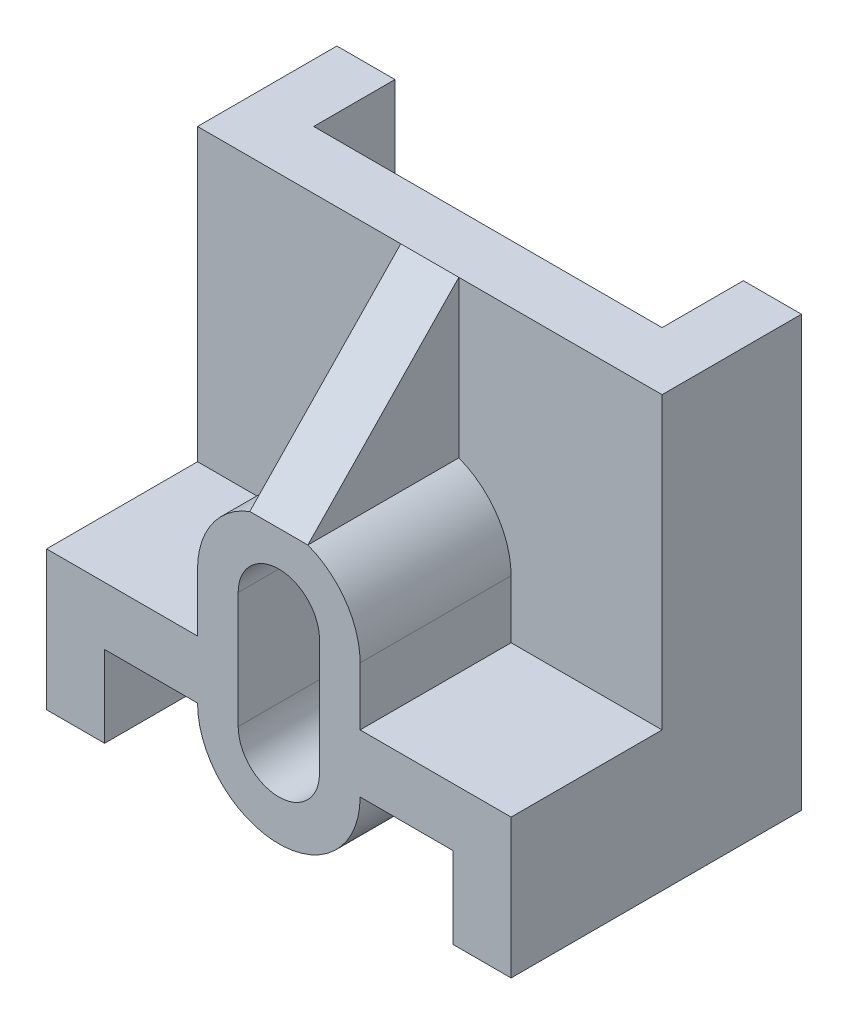
ISO-10303-21;
HEADER;
FILE_DESCRIPTION(('STEP AP214'),'2;1');
FILE_NAME('part.step','',(''),(''),'','','');
FILE_SCHEMA(('AUTOMOTIVE_DESIGN { 1 0 10303 214 1 1 1 1 }'));
ENDSEC;
DATA;
#1=APPLICATION_CONTEXT('core data for automotive mechanical design processes');
#2=APPLICATION_PROTOCOL_DEFINITION('international standard','automotive_design',2000,#1);
#3=PRODUCT_CONTEXT('',#1,'mechanical');
#4=PRODUCT('Part','Part','',(#3));
#5=PRODUCT_RELATED_PRODUCT_CATEGORY('part','',(#4));
#6=PRODUCT_DEFINITION_FORMATION('','',#4);
#7=PRODUCT_DEFINITION_CONTEXT('part definition',#1,'design');
#8=PRODUCT_DEFINITION('design','',#6,#7);
#9=PRODUCT_DEFINITION_SHAPE('','',#8);
#10=(LENGTH_UNIT() NAMED_UNIT(*) SI_UNIT(.MILLI.,.METRE.));
#11=(NAMED_UNIT(*) PLANE_ANGLE_UNIT() SI_UNIT($,.RADIAN.));
#12=(NAMED_UNIT(*) SI_UNIT($,.STERADIAN.) SOLID_ANGLE_UNIT());
#13=UNCERTAINTY_MEASURE_WITH_UNIT(LENGTH_MEASURE(1.E-05),#10,'distance_accuracy_value','');
#14=(GEOMETRIC_REPRESENTATION_CONTEXT(3) GLOBAL_UNCERTAINTY_ASSIGNED_CONTEXT((#13)) GLOBAL_UNIT_ASSIGNED_CONTEXT((#10,
#11,#12)) REPRESENTATION_CONTEXT('',''));
#15=CARTESIAN_POINT('',(0.,0.,0.));
#16=DIRECTION('',(0.,0.,1.));
#17=DIRECTION('',(1.,0.,0.));
#18=AXIS2_PLACEMENT_3D('',#15,#16,#17);
#19=CARTESIAN_POINT('',(0.,0.,0.));
#20=DIRECTION('',(0.,0.,-1.));
#21=DIRECTION('',(-1.,0.,0.));
#22=AXIS2_PLACEMENT_3D('',#19,#20,#21);
#23=PLANE('',#22);
#24=DIRECTION('',(0.,1.,0.));
#25=VECTOR('',#24,1.);
#26=CARTESIAN_POINT('',(47.,-10.,0.));
#27=LINE('',#26,#25);
#28=CARTESIAN_POINT('',(47.,-10.,0.));
#29=VERTEX_POINT('',#28);
#30=CARTESIAN_POINT('',(47.,10.,0.));
#31=VERTEX_POINT('',#30);
#32=EDGE_CURVE('E247',#29,#31,#27,.T.);
#33=ORIENTED_EDGE('',*,*,#32,.F.);
#34=CARTESIAN_POINT('',(40.,-10.,0.));
#35=DIRECTION('',(0.,0.,1.));
#36=DIRECTION('',(1.,0.,0.));
#37=AXIS2_PLACEMENT_3D('',#34,#35,#36);
#38=CIRCLE('',#37,7.);
#39=CARTESIAN_POINT('',(33.,-10.,0.));
#40=VERTEX_POINT('',#39);
#41=EDGE_CURVE('E64',#40,#29,#38,.T.);
#42=ORIENTED_EDGE('',*,*,#41,.F.);
#43=DIRECTION('',(0.,-1.,0.));
#44=VECTOR('',#43,1.);
#45=CARTESIAN_POINT('',(33.,-10.,0.));
#46=LINE('',#45,#44);
#47=CARTESIAN_POINT('',(33.,10.,0.));
#48=VERTEX_POINT('',#47);
#49=EDGE_CURVE('E258',#48,#40,#46,.T.);
#50=ORIENTED_EDGE('',*,*,#49,.F.);
#51=CARTESIAN_POINT('',(40.,10.,0.));
#52=DIRECTION('',(0.,0.,1.));
#53=DIRECTION('',(1.,0.,0.));
#54=AXIS2_PLACEMENT_3D('',#51,#52,#53);
#55=CIRCLE('',#54,7.);
#56=EDGE_CURVE('E251',#31,#48,#55,.T.);
#57=ORIENTED_EDGE('',*,*,#56,.F.);
#58=EDGE_LOOP('',(#33,#42,#50,#57));
#59=FACE_BOUND('',#58,.T.);
#60=DIRECTION('',(1.,0.,0.));
#61=VECTOR('',#60,1.);
#62=CARTESIAN_POINT('',(-114.874947873219,23.076696830622,0.));
#63=LINE('',#62,#61);
#64=CARTESIAN_POINT('',(35.,23.076696830622,0.));
#65=VERTEX_POINT('',#64);
#66=CARTESIAN_POINT('',(45.,23.076696830622,0.));
#67=VERTEX_POINT('',#66);
#68=EDGE_CURVE('E53',#65,#67,#63,.T.);
#69=ORIENTED_EDGE('',*,*,#68,.F.);
#70=CARTESIAN_POINT('',(40.,10.,0.));
#71=DIRECTION('',(0.,0.,1.));
#72=DIRECTION('',(1.,0.,0.));
#73=AXIS2_PLACEMENT_3D('',#70,#71,#72);
#74=CIRCLE('',#73,14.);
#75=CARTESIAN_POINT('',(26.,10.,0.));
#76=VERTEX_POINT('',#75);
#77=EDGE_CURVE('E282',#65,#76,#74,.T.);
#78=ORIENTED_EDGE('',*,*,#77,.T.);
#79=DIRECTION('',(0.,-1.,0.));
#80=VECTOR('',#79,1.);
#81=CARTESIAN_POINT('',(26.,10.,0.));
#82=LINE('',#81,#80);
#83=CARTESIAN_POINT('',(26.,0.,0.));
#84=VERTEX_POINT('',#83);
#85=EDGE_CURVE('E278',#76,#84,#82,.T.);
#86=ORIENTED_EDGE('',*,*,#85,.T.);
#87=DIRECTION('',(-1.,0.,0.));
#88=VECTOR('',#87,1.);
#89=CARTESIAN_POINT('',(0.,0.,0.));
#90=LINE('',#89,#88);
#91=CARTESIAN_POINT('',(0.,0.,0.));
#92=VERTEX_POINT('',#91);
#93=EDGE_CURVE('E374',#84,#92,#90,.T.);
#94=ORIENTED_EDGE('',*,*,#93,.T.);
#95=DIRECTION('',(0.,-1.,0.));
#96=VECTOR('',#95,1.);
#97=CARTESIAN_POINT('',(0.,-24.,0.));
#98=LINE('',#97,#96);
#99=CARTESIAN_POINT('',(0.,-24.,0.));
#100=VERTEX_POINT('',#99);
#101=EDGE_CURVE('E333',#92,#100,#98,.T.);
#102=ORIENTED_EDGE('',*,*,#101,.T.);
#103=DIRECTION('',(1.,0.,0.));
#104=VECTOR('',#103,1.);
#105=CARTESIAN_POINT('',(9.99999999999999,-24.,0.));
#106=LINE('',#105,#104);
#107=CARTESIAN_POINT('',(9.99999999999999,-24.,0.));
#108=VERTEX_POINT('',#107);
#109=EDGE_CURVE('E358',#100,#108,#106,.T.);
#110=ORIENTED_EDGE('',*,*,#109,.T.);
#111=DIRECTION('',(0.,1.,0.));
#112=VECTOR('',#111,1.);
#113=CARTESIAN_POINT('',(9.99999999999999,-10.,0.));
#114=LINE('',#113,#112);
#115=CARTESIAN_POINT('',(9.99999999999999,-10.,0.));
#116=VERTEX_POINT('',#115);
#117=EDGE_CURVE('E359',#108,#116,#114,.T.);
#118=ORIENTED_EDGE('',*,*,#117,.T.);
#119=DIRECTION('',(1.,0.,0.));
#120=VECTOR('',#119,1.);
#121=CARTESIAN_POINT('',(70.,-10.,0.));
#122=LINE('',#121,#120);
#123=CARTESIAN_POINT('',(26.,-10.,0.));
#124=VERTEX_POINT('',#123);
#125=EDGE_CURVE('E361',#116,#124,#122,.T.);
#126=ORIENTED_EDGE('',*,*,#125,.T.);
#127=CARTESIAN_POINT('',(40.,-10.,0.));
#128=DIRECTION('',(0.,0.,1.));
#129=DIRECTION('',(1.,0.,0.));
#130=AXIS2_PLACEMENT_3D('',#127,#128,#129);
#131=CIRCLE('',#130,14.);
#132=CARTESIAN_POINT('',(54.,-10.,0.));
#133=VERTEX_POINT('',#132);
#134=EDGE_CURVE('E281',#124,#133,#131,.T.);
#135=ORIENTED_EDGE('',*,*,#134,.T.);
#136=CARTESIAN_POINT('',(70.,-10.,0.));
#137=VERTEX_POINT('',#136);
#138=EDGE_CURVE('E362',#133,#137,#122,.T.);
#139=ORIENTED_EDGE('',*,*,#138,.T.);
#140=DIRECTION('',(0.,-1.,0.));
#141=VECTOR('',#140,1.);
#142=CARTESIAN_POINT('',(70.,-24.,0.));
#143=LINE('',#142,#141);
#144=CARTESIAN_POINT('',(70.,-24.,0.));
#145=VERTEX_POINT('',#144);
#146=EDGE_CURVE('E368',#137,#145,#143,.T.);
#147=ORIENTED_EDGE('',*,*,#146,.T.);
#148=DIRECTION('',(1.,0.,0.));
#149=VECTOR('',#148,1.);
#150=CARTESIAN_POINT('',(80.,-24.,0.));
#151=LINE('',#150,#149);
#152=CARTESIAN_POINT('',(80.,-24.,0.));
#153=VERTEX_POINT('',#152);
#154=EDGE_CURVE('E369',#145,#153,#151,.T.);
#155=ORIENTED_EDGE('',*,*,#154,.T.);
#156=DIRECTION('',(0.,1.,0.));
#157=VECTOR('',#156,1.);
#158=CARTESIAN_POINT('',(80.,0.,0.));
#159=LINE('',#158,#157);
#160=CARTESIAN_POINT('',(80.,0.,0.));
#161=VERTEX_POINT('',#160);
#162=EDGE_CURVE('E375',#153,#161,#159,.T.);
#163=ORIENTED_EDGE('',*,*,#162,.T.);
#164=CARTESIAN_POINT('',(54.,0.,0.));
#165=VERTEX_POINT('',#164);
#166=EDGE_CURVE('E338',#161,#165,#90,.T.);
#167=ORIENTED_EDGE('',*,*,#166,.T.);
#168=DIRECTION('',(0.,1.,0.));
#169=VECTOR('',#168,1.);
#170=CARTESIAN_POINT('',(54.,10.,0.));
#171=LINE('',#170,#169);
#172=CARTESIAN_POINT('',(54.,10.,0.));
#173=VERTEX_POINT('',#172);
#174=EDGE_CURVE('E288',#165,#173,#171,.T.);
#175=ORIENTED_EDGE('',*,*,#174,.T.);
#176=EDGE_CURVE('E279',#173,#67,#74,.T.);
#177=ORIENTED_EDGE('',*,*,#176,.T.);
#178=EDGE_LOOP('',(#69,#78,#86,#94,#102,#110,#118,#126,#135,#139,#147,#155,#163,#167,#175,#177));
#179=FACE_BOUND('',#178,.T.);
#180=ADVANCED_FACE('F39',(#59,#179),#23,.F.);
#181=CARTESIAN_POINT('',(0.,50.,0.));
#182=DIRECTION('',(0.,1.,0.));
#183=DIRECTION('',(0.,0.,1.));
#184=AXIS2_PLACEMENT_3D('',#181,#182,#183);
#185=PLANE('',#184);
#186=DIRECTION('',(1.,0.,0.));
#187=VECTOR('',#186,1.);
#188=CARTESIAN_POINT('',(0.,50.,-26.));
#189=LINE('',#188,#187);
#190=CARTESIAN_POINT('',(0.,50.,-26.));
#191=VERTEX_POINT('',#190);
#192=CARTESIAN_POINT('',(35.,50.,-26.));
#193=VERTEX_POINT('',#192);
#194=EDGE_CURVE('E227',#191,#193,#189,.T.);
#195=ORIENTED_EDGE('',*,*,#194,.T.);
#196=DIRECTION('',(1.,0.,0.));
#197=VECTOR('',#196,1.);
#198=CARTESIAN_POINT('',(-114.874947873219,50.,-26.));
#199=LINE('',#198,#197);
#200=CARTESIAN_POINT('',(45.,50.,-26.));
#201=VERTEX_POINT('',#200);
#202=EDGE_CURVE('E240',#193,#201,#199,.T.);
#203=ORIENTED_EDGE('',*,*,#202,.T.);
#204=CARTESIAN_POINT('',(80.,50.,-26.));
#205=VERTEX_POINT('',#204);
#206=EDGE_CURVE('E212',#201,#205,#189,.T.);
#207=ORIENTED_EDGE('',*,*,#206,.T.);
#208=DIRECTION('',(0.,0.,-1.));
#209=VECTOR('',#208,1.);
#210=CARTESIAN_POINT('',(80.,50.,-50.));
#211=LINE('',#210,#209);
#212=CARTESIAN_POINT('',(80.,50.,-50.));
#213=VERTEX_POINT('',#212);
#214=EDGE_CURVE('E323',#205,#213,#211,.T.);
#215=ORIENTED_EDGE('',*,*,#214,.T.);
#216=DIRECTION('',(-1.,0.,0.));
#217=VECTOR('',#216,1.);
#218=CARTESIAN_POINT('',(0.,50.,-50.));
#219=LINE('',#218,#217);
#220=CARTESIAN_POINT('',(70.,50.,-50.));
#221=VERTEX_POINT('',#220);
#222=EDGE_CURVE('E326',#213,#221,#219,.T.);
#223=ORIENTED_EDGE('',*,*,#222,.T.);
#224=DIRECTION('',(0.,0.,-1.));
#225=VECTOR('',#224,1.);
#226=CARTESIAN_POINT('',(70.,50.,-50.));
#227=LINE('',#226,#225);
#228=CARTESIAN_POINT('',(70.,50.,-36.));
#229=VERTEX_POINT('',#228);
#230=EDGE_CURVE('E306',#229,#221,#227,.T.);
#231=ORIENTED_EDGE('',*,*,#230,.F.);
#232=DIRECTION('',(1.,0.,0.));
#233=VECTOR('',#232,1.);
#234=CARTESIAN_POINT('',(10.,50.,-36.));
#235=LINE('',#234,#233);
#236=CARTESIAN_POINT('',(10.,50.,-36.));
#237=VERTEX_POINT('',#236);
#238=EDGE_CURVE('E302',#237,#229,#235,.T.);
#239=ORIENTED_EDGE('',*,*,#238,.F.);
#240=DIRECTION('',(0.,0.,1.));
#241=VECTOR('',#240,1.);
#242=CARTESIAN_POINT('',(9.99999999999999,50.,-50.));
#243=LINE('',#242,#241);
#244=CARTESIAN_POINT('',(9.99999999999999,50.,-50.));
#245=VERTEX_POINT('',#244);
#246=EDGE_CURVE('E301',#245,#237,#243,.T.);
#247=ORIENTED_EDGE('',*,*,#246,.F.);
#248=CARTESIAN_POINT('',(0.,50.,-50.));
#249=VERTEX_POINT('',#248);
#250=EDGE_CURVE('E324',#245,#249,#219,.T.);
#251=ORIENTED_EDGE('',*,*,#250,.T.);
#252=DIRECTION('',(0.,0.,1.));
#253=VECTOR('',#252,1.);
#254=CARTESIAN_POINT('',(0.,50.,-50.));
#255=LINE('',#254,#253);
#256=EDGE_CURVE('E229',#249,#191,#255,.T.);
#257=ORIENTED_EDGE('',*,*,#256,.T.);
#258=EDGE_LOOP('',(#195,#203,#207,#215,#223,#231,#239,#247,#251,#257));
#259=FACE_BOUND('',#258,.T.);
#260=ADVANCED_FACE('F236',(#259),#185,.T.);
#261=CARTESIAN_POINT('',(35.,50.,0.));
#262=DIRECTION('',(1.,0.,0.));
#263=DIRECTION('',(0.,1.,0.));
#264=AXIS2_PLACEMENT_3D('',#261,#262,#263);
#265=PLANE('',#264);
#266=DIRECTION('',(0.,0.719333547480298,-0.694664845425051));
#267=VECTOR('',#266,1.);
#268=CARTESIAN_POINT('',(35.,50.,-26.));
#269=LINE('',#268,#267);
#270=EDGE_CURVE('E241',#65,#193,#269,.T.);
#271=ORIENTED_EDGE('',*,*,#270,.T.);
#272=DIRECTION('',(0.,-1.,0.));
#273=VECTOR('',#272,1.);
#274=CARTESIAN_POINT('',(35.,50.,-26.));
#275=LINE('',#274,#273);
#276=CARTESIAN_POINT('',(35.,23.076696830622,-26.));
#277=VERTEX_POINT('',#276);
#278=EDGE_CURVE('E231',#193,#277,#275,.T.);
#279=ORIENTED_EDGE('',*,*,#278,.T.);
#280=DIRECTION('',(0.,0.,1.));
#281=VECTOR('',#280,1.);
#282=CARTESIAN_POINT('',(35.,23.076696830622,-26.));
#283=LINE('',#282,#281);
#284=EDGE_CURVE('E50',#65,#277,#283,.F.);
#285=ORIENTED_EDGE('',*,*,#284,.F.);
#286=EDGE_LOOP('',(#271,#279,#285));
#287=FACE_BOUND('',#286,.T.);
#288=ADVANCED_FACE('F499',(#287),#265,.F.);
#289=CARTESIAN_POINT('',(45.,50.,0.));
#290=DIRECTION('',(-1.,0.,0.));
#291=DIRECTION('',(0.,0.,1.));
#292=AXIS2_PLACEMENT_3D('',#289,#290,#291);
#293=PLANE('',#292);
#294=DIRECTION('',(0.,0.719333547480298,-0.694664845425051));
#295=VECTOR('',#294,1.);
#296=CARTESIAN_POINT('',(45.,37.0079110831942,-13.4534595657953));
#297=LINE('',#296,#295);
#298=EDGE_CURVE('E11',#67,#201,#297,.T.);
#299=ORIENTED_EDGE('',*,*,#298,.F.);
#300=DIRECTION('',(0.,0.,1.));
#301=VECTOR('',#300,1.);
#302=CARTESIAN_POINT('',(45.,23.076696830622,-26.));
#303=LINE('',#302,#301);
#304=CARTESIAN_POINT('',(45.,23.076696830622,-26.));
#305=VERTEX_POINT('',#304);
#306=EDGE_CURVE('E235',#305,#67,#303,.T.);
#307=ORIENTED_EDGE('',*,*,#306,.F.);
#308=DIRECTION('',(0.,1.,0.));
#309=VECTOR('',#308,1.);
#310=CARTESIAN_POINT('',(45.,50.,-26.));
#311=LINE('',#310,#309);
#312=EDGE_CURVE('E217',#305,#201,#311,.T.);
#313=ORIENTED_EDGE('',*,*,#312,.T.);
#314=EDGE_LOOP('',(#299,#307,#313));
#315=FACE_BOUND('',#314,.T.);
#316=ADVANCED_FACE('F228',(#315),#293,.F.);
#317=CARTESIAN_POINT('',(0.,50.,-26.));
#318=DIRECTION('',(0.,0.,-1.));
#319=DIRECTION('',(-1.,0.,0.));
#320=AXIS2_PLACEMENT_3D('',#317,#318,#319);
#321=PLANE('',#320);
#322=ORIENTED_EDGE('',*,*,#278,.F.);
#323=ORIENTED_EDGE('',*,*,#194,.F.);
#324=DIRECTION('',(0.,-1.,0.));
#325=VECTOR('',#324,1.);
#326=CARTESIAN_POINT('',(0.,50.,-26.));
#327=LINE('',#326,#325);
#328=CARTESIAN_POINT('',(0.,0.,-26.));
#329=VERTEX_POINT('',#328);
#330=EDGE_CURVE('E335',#191,#329,#327,.T.);
#331=ORIENTED_EDGE('',*,*,#330,.T.);
#332=DIRECTION('',(1.,0.,0.));
#333=VECTOR('',#332,1.);
#334=CARTESIAN_POINT('',(0.,0.,-26.));
#335=LINE('',#334,#333);
#336=CARTESIAN_POINT('',(26.,0.,-26.));
#337=VERTEX_POINT('',#336);
#338=EDGE_CURVE('E321',#329,#337,#335,.T.);
#339=ORIENTED_EDGE('',*,*,#338,.T.);
#340=DIRECTION('',(0.,-1.,0.));
#341=VECTOR('',#340,1.);
#342=CARTESIAN_POINT('',(26.,10.,-26.));
#343=LINE('',#342,#341);
#344=CARTESIAN_POINT('',(26.,10.,-26.));
#345=VERTEX_POINT('',#344);
#346=EDGE_CURVE('E271',#345,#337,#343,.T.);
#347=ORIENTED_EDGE('',*,*,#346,.F.);
#348=CARTESIAN_POINT('',(40.,10.,-26.));
#349=DIRECTION('',(0.,0.,1.));
#350=DIRECTION('',(1.,0.,0.));
#351=AXIS2_PLACEMENT_3D('',#348,#349,#350);
#352=CIRCLE('',#351,14.);
#353=EDGE_CURVE('E275',#277,#345,#352,.T.);
#354=ORIENTED_EDGE('',*,*,#353,.F.);
#355=EDGE_LOOP('',(#322,#323,#331,#339,#347,#354));
#356=FACE_BOUND('',#355,.T.);
#357=ADVANCED_FACE('F424',(#356),#321,.F.);
#358=ORIENTED_EDGE('',*,*,#312,.F.);
#359=CARTESIAN_POINT('',(54.,10.,-26.));
#360=VERTEX_POINT('',#359);
#361=EDGE_CURVE('E267',#360,#305,#352,.T.);
#362=ORIENTED_EDGE('',*,*,#361,.F.);
#363=DIRECTION('',(0.,-1.,0.));
#364=VECTOR('',#363,1.);
#365=CARTESIAN_POINT('',(54.,50.,-26.));
#366=LINE('',#365,#364);
#367=CARTESIAN_POINT('',(54.,0.,-26.));
#368=VERTEX_POINT('',#367);
#369=EDGE_CURVE('E381',#360,#368,#366,.T.);
#370=ORIENTED_EDGE('',*,*,#369,.T.);
#371=CARTESIAN_POINT('',(80.,0.,-26.));
#372=VERTEX_POINT('',#371);
#373=EDGE_CURVE('E319',#368,#372,#335,.T.);
#374=ORIENTED_EDGE('',*,*,#373,.T.);
#375=DIRECTION('',(0.,-1.,0.));
#376=VECTOR('',#375,1.);
#377=CARTESIAN_POINT('',(80.,50.,-26.));
#378=LINE('',#377,#376);
#379=EDGE_CURVE('E222',#205,#372,#378,.T.);
#380=ORIENTED_EDGE('',*,*,#379,.F.);
#381=ORIENTED_EDGE('',*,*,#206,.F.);
#382=EDGE_LOOP('',(#358,#362,#370,#374,#380,#381));
#383=FACE_BOUND('',#382,.T.);
#384=ADVANCED_FACE('F216',(#383),#321,.F.);
#385=CARTESIAN_POINT('',(40.,10.,-26.));
#386=DIRECTION('',(0.,0.,1.));
#387=DIRECTION('',(1.,0.,0.));
#388=AXIS2_PLACEMENT_3D('',#385,#386,#387);
#389=CYLINDRICAL_SURFACE('',#388,14.);
#390=ORIENTED_EDGE('',*,*,#77,.F.);
#391=ORIENTED_EDGE('',*,*,#284,.T.);
#392=ORIENTED_EDGE('',*,*,#353,.T.);
#393=DIRECTION('',(0.,0.,1.));
#394=VECTOR('',#393,1.);
#395=CARTESIAN_POINT('',(26.,10.,-26.));
#396=LINE('',#395,#394);
#397=EDGE_CURVE('E280',#345,#76,#396,.T.);
#398=ORIENTED_EDGE('',*,*,#397,.T.);
#399=EDGE_LOOP('',(#390,#391,#392,#398));
#400=FACE_BOUND('',#399,.T.);
#401=ADVANCED_FACE('F416',(#400),#389,.T.);
#402=ORIENTED_EDGE('',*,*,#361,.T.);
#403=ORIENTED_EDGE('',*,*,#306,.T.);
#404=ORIENTED_EDGE('',*,*,#176,.F.);
#405=DIRECTION('',(0.,0.,1.));
#406=VECTOR('',#405,1.);
#407=CARTESIAN_POINT('',(54.,10.,-26.));
#408=LINE('',#407,#406);
#409=EDGE_CURVE('E286',#360,#173,#408,.T.);
#410=ORIENTED_EDGE('',*,*,#409,.F.);
#411=EDGE_LOOP('',(#402,#403,#404,#410));
#412=FACE_BOUND('',#411,.T.);
#413=ADVANCED_FACE('F544',(#412),#389,.T.);
#414=CARTESIAN_POINT('',(70.,-10.,-50.));
#415=DIRECTION('',(0.,-1.,0.));
#416=DIRECTION('',(0.,0.,-1.));
#417=AXIS2_PLACEMENT_3D('',#414,#415,#416);
#418=PLANE('',#417);
#419=DIRECTION('',(0.,0.,1.));
#420=VECTOR('',#419,1.);
#421=CARTESIAN_POINT('',(33.,-10.,-50.));
#422=LINE('',#421,#420);
#423=CARTESIAN_POINT('',(33.,-10.,-36.));
#424=VERTEX_POINT('',#423);
#425=CARTESIAN_POINT('',(33.,-10.,-26.));
#426=VERTEX_POINT('',#425);
#427=EDGE_CURVE('E265',#424,#426,#422,.T.);
#428=ORIENTED_EDGE('',*,*,#427,.T.);
#429=DIRECTION('',(-1.,0.,0.));
#430=VECTOR('',#429,1.);
#431=CARTESIAN_POINT('',(70.,-10.,-26.));
#432=LINE('',#431,#430);
#433=CARTESIAN_POINT('',(26.,-10.,-26.));
#434=VERTEX_POINT('',#433);
#435=EDGE_CURVE('E396',#426,#434,#432,.T.);
#436=ORIENTED_EDGE('',*,*,#435,.T.);
#437=DIRECTION('',(0.,0.,1.));
#438=VECTOR('',#437,1.);
#439=CARTESIAN_POINT('',(26.,-10.,-26.));
#440=LINE('',#439,#438);
#441=EDGE_CURVE('E293',#434,#124,#440,.T.);
#442=ORIENTED_EDGE('',*,*,#441,.T.);
#443=ORIENTED_EDGE('',*,*,#125,.F.);
#444=DIRECTION('',(0.,0.,1.));
#445=VECTOR('',#444,1.);
#446=CARTESIAN_POINT('',(9.99999999999999,-10.,-50.));
#447=LINE('',#446,#445);
#448=CARTESIAN_POINT('',(10.,-10.,-36.));
#449=VERTEX_POINT('',#448);
#450=EDGE_CURVE('E392',#449,#116,#447,.T.);
#451=ORIENTED_EDGE('',*,*,#450,.F.);
#452=DIRECTION('',(-1.,0.,0.));
#453=VECTOR('',#452,1.);
#454=CARTESIAN_POINT('',(70.,-10.,-36.));
#455=LINE('',#454,#453);
#456=EDGE_CURVE('E314',#424,#449,#455,.T.);
#457=ORIENTED_EDGE('',*,*,#456,.F.);
#458=EDGE_LOOP('',(#428,#436,#442,#443,#451,#457));
#459=FACE_BOUND('',#458,.T.);
#460=ADVANCED_FACE('F437',(#459),#418,.T.);
#461=CARTESIAN_POINT('',(0.,0.,-50.));
#462=DIRECTION('',(0.,1.,0.));
#463=DIRECTION('',(0.,0.,1.));
#464=AXIS2_PLACEMENT_3D('',#461,#462,#463);
#465=PLANE('',#464);
#466=DIRECTION('',(0.,0.,-1.));
#467=VECTOR('',#466,1.);
#468=CARTESIAN_POINT('',(54.,0.,-50.));
#469=LINE('',#468,#467);
#470=EDGE_CURVE('E303',#165,#368,#469,.T.);
#471=ORIENTED_EDGE('',*,*,#470,.F.);
#472=ORIENTED_EDGE('',*,*,#166,.F.);
#473=DIRECTION('',(0.,0.,1.));
#474=VECTOR('',#473,1.);
#475=CARTESIAN_POINT('',(80.,0.,-50.));
#476=LINE('',#475,#474);
#477=EDGE_CURVE('E385',#372,#161,#476,.T.);
#478=ORIENTED_EDGE('',*,*,#477,.F.);
#479=ORIENTED_EDGE('',*,*,#373,.F.);
#480=EDGE_LOOP('',(#471,#472,#478,#479));
#481=FACE_BOUND('',#480,.T.);
#482=ADVANCED_FACE('F510',(#481),#465,.T.);
#483=CARTESIAN_POINT('',(0.,0.,-50.));
#484=DIRECTION('',(0.,0.,-1.));
#485=DIRECTION('',(-1.,0.,0.));
#486=AXIS2_PLACEMENT_3D('',#483,#484,#485);
#487=PLANE('',#486);
#488=ORIENTED_EDGE('',*,*,#250,.F.);
#489=DIRECTION('',(0.,1.,0.));
#490=VECTOR('',#489,1.);
#491=CARTESIAN_POINT('',(9.99999999999999,-10.,-50.));
#492=LINE('',#491,#490);
#493=CARTESIAN_POINT('',(9.99999999999999,-24.,-50.));
#494=VERTEX_POINT('',#493);
#495=EDGE_CURVE('E341',#494,#245,#492,.T.);
#496=ORIENTED_EDGE('',*,*,#495,.F.);
#497=DIRECTION('',(1.,0.,0.));
#498=VECTOR('',#497,1.);
#499=CARTESIAN_POINT('',(9.99999999999999,-24.,-50.));
#500=LINE('',#499,#498);
#501=CARTESIAN_POINT('',(0.,-24.,-50.));
#502=VERTEX_POINT('',#501);
#503=EDGE_CURVE('E336',#502,#494,#500,.T.);
#504=ORIENTED_EDGE('',*,*,#503,.F.);
#505=DIRECTION('',(0.,-1.,0.));
#506=VECTOR('',#505,1.);
#507=CARTESIAN_POINT('',(0.,-24.,-50.));
#508=LINE('',#507,#506);
#509=EDGE_CURVE('E337',#249,#502,#508,.T.);
#510=ORIENTED_EDGE('',*,*,#509,.F.);
#511=EDGE_LOOP('',(#488,#496,#504,#510));
#512=FACE_BOUND('',#511,.T.);
#513=ADVANCED_FACE('F527',(#512),#487,.T.);
#514=CARTESIAN_POINT('',(0.,-24.,-50.));
#515=DIRECTION('',(-1.,0.,0.));
#516=DIRECTION('',(0.,0.,1.));
#517=AXIS2_PLACEMENT_3D('',#514,#515,#516);
#518=PLANE('',#517);
#519=ORIENTED_EDGE('',*,*,#101,.F.);
#520=DIRECTION('',(0.,0.,1.));
#521=VECTOR('',#520,1.);
#522=CARTESIAN_POINT('',(0.,0.,-50.));
#523=LINE('',#522,#521);
#524=EDGE_CURVE('E378',#329,#92,#523,.T.);
#525=ORIENTED_EDGE('',*,*,#524,.F.);
#526=ORIENTED_EDGE('',*,*,#330,.F.);
#527=ORIENTED_EDGE('',*,*,#256,.F.);
#528=ORIENTED_EDGE('',*,*,#509,.T.);
#529=DIRECTION('',(0.,0.,1.));
#530=VECTOR('',#529,1.);
#531=CARTESIAN_POINT('',(0.,-24.,-50.));
#532=LINE('',#531,#530);
#533=EDGE_CURVE('E355',#502,#100,#532,.T.);
#534=ORIENTED_EDGE('',*,*,#533,.T.);
#535=EDGE_LOOP('',(#519,#525,#526,#527,#528,#534));
#536=FACE_BOUND('',#535,.T.);
#537=ADVANCED_FACE('F41',(#536),#518,.T.);
#538=DIRECTION('',(0.,0.,1.));
#539=VECTOR('',#538,1.);
#540=CARTESIAN_POINT('',(26.,0.,-50.));
#541=LINE('',#540,#539);
#542=EDGE_CURVE('E292',#337,#84,#541,.T.);
#543=ORIENTED_EDGE('',*,*,#542,.F.);
#544=ORIENTED_EDGE('',*,*,#338,.F.);
#545=ORIENTED_EDGE('',*,*,#524,.T.);
#546=ORIENTED_EDGE('',*,*,#93,.F.);
#547=EDGE_LOOP('',(#543,#544,#545,#546));
#548=FACE_BOUND('',#547,.T.);
#549=ADVANCED_FACE('F431',(#548),#465,.T.);
#550=CARTESIAN_POINT('',(80.,0.,-50.));
#551=DIRECTION('',(1.,0.,0.));
#552=DIRECTION('',(0.,0.,-1.));
#553=AXIS2_PLACEMENT_3D('',#550,#551,#552);
#554=PLANE('',#553);
#555=ORIENTED_EDGE('',*,*,#162,.F.);
#556=DIRECTION('',(0.,0.,1.));
#557=VECTOR('',#556,1.);
#558=CARTESIAN_POINT('',(80.,-24.,-50.));
#559=LINE('',#558,#557);
#560=CARTESIAN_POINT('',(80.,-24.,-50.));
#561=VERTEX_POINT('',#560);
#562=EDGE_CURVE('E383',#561,#153,#559,.T.);
#563=ORIENTED_EDGE('',*,*,#562,.F.);
#564=DIRECTION('',(0.,1.,0.));
#565=VECTOR('',#564,1.);
#566=CARTESIAN_POINT('',(80.,0.,-50.));
#567=LINE('',#566,#565);
#568=EDGE_CURVE('E352',#561,#213,#567,.T.);
#569=ORIENTED_EDGE('',*,*,#568,.T.);
#570=ORIENTED_EDGE('',*,*,#214,.F.);
#571=ORIENTED_EDGE('',*,*,#379,.T.);
#572=ORIENTED_EDGE('',*,*,#477,.T.);
#573=EDGE_LOOP('',(#555,#563,#569,#570,#571,#572));
#574=FACE_BOUND('',#573,.T.);
#575=ADVANCED_FACE('F508',(#574),#554,.T.);
#576=CARTESIAN_POINT('',(80.,-24.,-50.));
#577=DIRECTION('',(0.,-1.,0.));
#578=DIRECTION('',(0.,0.,-1.));
#579=AXIS2_PLACEMENT_3D('',#576,#577,#578);
#580=PLANE('',#579);
#581=ORIENTED_EDGE('',*,*,#154,.F.);
#582=DIRECTION('',(0.,0.,1.));
#583=VECTOR('',#582,1.);
#584=CARTESIAN_POINT('',(70.,-24.,-50.));
#585=LINE('',#584,#583);
#586=CARTESIAN_POINT('',(70.,-24.,-50.));
#587=VERTEX_POINT('',#586);
#588=EDGE_CURVE('E387',#587,#145,#585,.T.);
#589=ORIENTED_EDGE('',*,*,#588,.F.);
#590=DIRECTION('',(1.,0.,0.));
#591=VECTOR('',#590,1.);
#592=CARTESIAN_POINT('',(80.,-24.,-50.));
#593=LINE('',#592,#591);
#594=EDGE_CURVE('E346',#587,#561,#593,.T.);
#595=ORIENTED_EDGE('',*,*,#594,.T.);
#596=ORIENTED_EDGE('',*,*,#562,.T.);
#597=EDGE_LOOP('',(#581,#589,#595,#596));
#598=FACE_BOUND('',#597,.T.);
#599=ADVANCED_FACE('F507',(#598),#580,.T.);
#600=CARTESIAN_POINT('',(70.,-24.,-50.));
#601=DIRECTION('',(-1.,0.,0.));
#602=DIRECTION('',(0.,0.,1.));
#603=AXIS2_PLACEMENT_3D('',#600,#601,#602);
#604=PLANE('',#603);
#605=DIRECTION('',(0.,0.,1.));
#606=VECTOR('',#605,1.);
#607=CARTESIAN_POINT('',(70.,-10.,-50.));
#608=LINE('',#607,#606);
#609=CARTESIAN_POINT('',(70.,-10.,-36.));
#610=VERTEX_POINT('',#609);
#611=EDGE_CURVE('E389',#610,#137,#608,.T.);
#612=ORIENTED_EDGE('',*,*,#611,.F.);
#613=DIRECTION('',(0.,1.,0.));
#614=VECTOR('',#613,1.);
#615=CARTESIAN_POINT('',(70.,-24.,-36.));
#616=LINE('',#615,#614);
#617=EDGE_CURVE('E315',#610,#229,#616,.T.);
#618=ORIENTED_EDGE('',*,*,#617,.T.);
#619=ORIENTED_EDGE('',*,*,#230,.T.);
#620=DIRECTION('',(0.,-1.,0.));
#621=VECTOR('',#620,1.);
#622=CARTESIAN_POINT('',(70.,-24.,-50.));
#623=LINE('',#622,#621);
#624=EDGE_CURVE('E342',#221,#587,#623,.T.);
#625=ORIENTED_EDGE('',*,*,#624,.T.);
#626=ORIENTED_EDGE('',*,*,#588,.T.);
#627=ORIENTED_EDGE('',*,*,#146,.F.);
#628=EDGE_LOOP('',(#612,#618,#619,#625,#626,#627));
#629=FACE_BOUND('',#628,.T.);
#630=ADVANCED_FACE('F473',(#629),#604,.T.);
#631=DIRECTION('',(0.,0.,1.));
#632=VECTOR('',#631,1.);
#633=CARTESIAN_POINT('',(47.,-10.,-50.));
#634=LINE('',#633,#632);
#635=CARTESIAN_POINT('',(47.,-10.,-36.));
#636=VERTEX_POINT('',#635);
#637=CARTESIAN_POINT('',(47.,-10.,-26.));
#638=VERTEX_POINT('',#637);
#639=EDGE_CURVE('E270',#636,#638,#634,.T.);
#640=ORIENTED_EDGE('',*,*,#639,.F.);
#641=EDGE_CURVE('E320',#610,#636,#455,.T.);
#642=ORIENTED_EDGE('',*,*,#641,.F.);
#643=ORIENTED_EDGE('',*,*,#611,.T.);
#644=ORIENTED_EDGE('',*,*,#138,.F.);
#645=DIRECTION('',(0.,0.,1.));
#646=VECTOR('',#645,1.);
#647=CARTESIAN_POINT('',(54.,-10.,-26.));
#648=LINE('',#647,#646);
#649=CARTESIAN_POINT('',(54.,-10.,-26.));
#650=VERTEX_POINT('',#649);
#651=EDGE_CURVE('E295',#650,#133,#648,.T.);
#652=ORIENTED_EDGE('',*,*,#651,.F.);
#653=EDGE_CURVE('E399',#650,#638,#432,.T.);
#654=ORIENTED_EDGE('',*,*,#653,.T.);
#655=EDGE_LOOP('',(#640,#642,#643,#644,#652,#654));
#656=FACE_BOUND('',#655,.T.);
#657=ADVANCED_FACE('F455',(#656),#418,.T.);
#658=CARTESIAN_POINT('',(9.99999999999999,-10.,-50.));
#659=DIRECTION('',(1.,0.,0.));
#660=DIRECTION('',(0.,0.,-1.));
#661=AXIS2_PLACEMENT_3D('',#658,#659,#660);
#662=PLANE('',#661);
#663=ORIENTED_EDGE('',*,*,#117,.F.);
#664=DIRECTION('',(0.,0.,1.));
#665=VECTOR('',#664,1.);
#666=CARTESIAN_POINT('',(9.99999999999999,-24.,-50.));
#667=LINE('',#666,#665);
#668=EDGE_CURVE('E395',#494,#108,#667,.T.);
#669=ORIENTED_EDGE('',*,*,#668,.F.);
#670=ORIENTED_EDGE('',*,*,#495,.T.);
#671=ORIENTED_EDGE('',*,*,#246,.T.);
#672=DIRECTION('',(0.,1.,0.));
#673=VECTOR('',#672,1.);
#674=CARTESIAN_POINT('',(10.,-24.,-36.));
#675=LINE('',#674,#673);
#676=EDGE_CURVE('E313',#449,#237,#675,.T.);
#677=ORIENTED_EDGE('',*,*,#676,.F.);
#678=ORIENTED_EDGE('',*,*,#450,.T.);
#679=EDGE_LOOP('',(#663,#669,#670,#671,#677,#678));
#680=FACE_BOUND('',#679,.T.);
#681=ADVANCED_FACE('F458',(#680),#662,.T.);
#682=CARTESIAN_POINT('',(9.99999999999999,-24.,-50.));
#683=DIRECTION('',(0.,-1.,0.));
#684=DIRECTION('',(0.,0.,-1.));
#685=AXIS2_PLACEMENT_3D('',#682,#683,#684);
#686=PLANE('',#685);
#687=ORIENTED_EDGE('',*,*,#109,.F.);
#688=ORIENTED_EDGE('',*,*,#533,.F.);
#689=ORIENTED_EDGE('',*,*,#503,.T.);
#690=ORIENTED_EDGE('',*,*,#668,.T.);
#691=EDGE_LOOP('',(#687,#688,#689,#690));
#692=FACE_BOUND('',#691,.T.);
#693=ADVANCED_FACE('F518',(#692),#686,.T.);
#694=ORIENTED_EDGE('',*,*,#624,.F.);
#695=ORIENTED_EDGE('',*,*,#222,.F.);
#696=ORIENTED_EDGE('',*,*,#568,.F.);
#697=ORIENTED_EDGE('',*,*,#594,.F.);
#698=EDGE_LOOP('',(#694,#695,#696,#697));
#699=FACE_BOUND('',#698,.T.);
#700=ADVANCED_FACE('F504',(#699),#487,.T.);
#701=CARTESIAN_POINT('',(10.,-24.,-36.));
#702=DIRECTION('',(0.,0.,1.));
#703=DIRECTION('',(1.,0.,0.));
#704=AXIS2_PLACEMENT_3D('',#701,#702,#703);
#705=PLANE('',#704);
#706=CARTESIAN_POINT('',(40.,10.,-36.));
#707=DIRECTION('',(0.,0.,1.));
#708=DIRECTION('',(1.,0.,0.));
#709=AXIS2_PLACEMENT_3D('',#706,#707,#708);
#710=CIRCLE('',#709,7.);
#711=CARTESIAN_POINT('',(47.,10.,-36.));
#712=VERTEX_POINT('',#711);
#713=CARTESIAN_POINT('',(33.,10.,-36.));
#714=VERTEX_POINT('',#713);
#715=EDGE_CURVE('E410',#712,#714,#710,.T.);
#716=ORIENTED_EDGE('',*,*,#715,.T.);
#717=DIRECTION('',(0.,-1.,0.));
#718=VECTOR('',#717,1.);
#719=CARTESIAN_POINT('',(33.,-24.,-36.));
#720=LINE('',#719,#718);
#721=EDGE_CURVE('E413',#714,#424,#720,.T.);
#722=ORIENTED_EDGE('',*,*,#721,.T.);
#723=ORIENTED_EDGE('',*,*,#456,.T.);
#724=ORIENTED_EDGE('',*,*,#676,.T.);
#725=ORIENTED_EDGE('',*,*,#238,.T.);
#726=ORIENTED_EDGE('',*,*,#617,.F.);
#727=ORIENTED_EDGE('',*,*,#641,.T.);
#728=DIRECTION('',(0.,1.,0.));
#729=VECTOR('',#728,1.);
#730=CARTESIAN_POINT('',(47.,-24.,-36.));
#731=LINE('',#730,#729);
#732=EDGE_CURVE('E403',#636,#712,#731,.T.);
#733=ORIENTED_EDGE('',*,*,#732,.T.);
#734=EDGE_LOOP('',(#716,#722,#723,#724,#725,#726,#727,#733));
#735=FACE_BOUND('',#734,.T.);
#736=ADVANCED_FACE('F468',(#735),#705,.F.);
#737=CARTESIAN_POINT('',(26.,10.,-26.));
#738=DIRECTION('',(-1.,0.,0.));
#739=DIRECTION('',(0.,0.,1.));
#740=AXIS2_PLACEMENT_3D('',#737,#738,#739);
#741=PLANE('',#740);
#742=ORIENTED_EDGE('',*,*,#346,.T.);
#743=ORIENTED_EDGE('',*,*,#542,.T.);
#744=ORIENTED_EDGE('',*,*,#85,.F.);
#745=ORIENTED_EDGE('',*,*,#397,.F.);
#746=EDGE_LOOP('',(#742,#743,#744,#745));
#747=FACE_BOUND('',#746,.T.);
#748=ADVANCED_FACE('F430',(#747),#741,.T.);
#749=CARTESIAN_POINT('',(54.,10.,-26.));
#750=DIRECTION('',(1.,0.,0.));
#751=DIRECTION('',(0.,0.,-1.));
#752=AXIS2_PLACEMENT_3D('',#749,#750,#751);
#753=PLANE('',#752);
#754=ORIENTED_EDGE('',*,*,#174,.F.);
#755=ORIENTED_EDGE('',*,*,#470,.T.);
#756=ORIENTED_EDGE('',*,*,#369,.F.);
#757=ORIENTED_EDGE('',*,*,#409,.T.);
#758=EDGE_LOOP('',(#754,#755,#756,#757));
#759=FACE_BOUND('',#758,.T.);
#760=ADVANCED_FACE('F559',(#759),#753,.T.);
#761=CARTESIAN_POINT('',(40.,-10.,-26.));
#762=DIRECTION('',(0.,0.,1.));
#763=DIRECTION('',(1.,0.,0.));
#764=AXIS2_PLACEMENT_3D('',#761,#762,#763);
#765=CYLINDRICAL_SURFACE('',#764,14.);
#766=ORIENTED_EDGE('',*,*,#134,.F.);
#767=ORIENTED_EDGE('',*,*,#441,.F.);
#768=CARTESIAN_POINT('',(40.,-10.,-26.));
#769=DIRECTION('',(0.,0.,1.));
#770=DIRECTION('',(1.,0.,0.));
#771=AXIS2_PLACEMENT_3D('',#768,#769,#770);
#772=CIRCLE('',#771,14.);
#773=EDGE_CURVE('E273',#434,#650,#772,.T.);
#774=ORIENTED_EDGE('',*,*,#773,.T.);
#775=ORIENTED_EDGE('',*,*,#651,.T.);
#776=EDGE_LOOP('',(#766,#767,#774,#775));
#777=FACE_BOUND('',#776,.T.);
#778=ADVANCED_FACE('F450',(#777),#765,.T.);
#779=CARTESIAN_POINT('',(40.,10.,-26.));
#780=DIRECTION('',(0.,0.,1.));
#781=DIRECTION('',(1.,0.,0.));
#782=AXIS2_PLACEMENT_3D('',#779,#780,#781);
#783=PLANE('',#782);
#784=ORIENTED_EDGE('',*,*,#435,.F.);
#785=CARTESIAN_POINT('',(40.,-10.,-26.));
#786=DIRECTION('',(0.,0.,1.));
#787=DIRECTION('',(1.,0.,0.));
#788=AXIS2_PLACEMENT_3D('',#785,#786,#787);
#789=CIRCLE('',#788,7.);
#790=EDGE_CURVE('E405',#426,#638,#789,.T.);
#791=ORIENTED_EDGE('',*,*,#790,.T.);
#792=ORIENTED_EDGE('',*,*,#653,.F.);
#793=ORIENTED_EDGE('',*,*,#773,.F.);
#794=EDGE_LOOP('',(#784,#791,#792,#793));
#795=FACE_BOUND('',#794,.T.);
#796=ADVANCED_FACE('F443',(#795),#783,.F.);
#797=CARTESIAN_POINT('',(33.,-10.,-50.));
#798=DIRECTION('',(-1.,0.,0.));
#799=DIRECTION('',(0.,0.,1.));
#800=AXIS2_PLACEMENT_3D('',#797,#798,#799);
#801=PLANE('',#800);
#802=DIRECTION('',(0.,0.,1.));
#803=VECTOR('',#802,1.);
#804=CARTESIAN_POINT('',(33.,10.,-50.));
#805=LINE('',#804,#803);
#806=EDGE_CURVE('E263',#714,#48,#805,.T.);
#807=ORIENTED_EDGE('',*,*,#806,.T.);
#808=ORIENTED_EDGE('',*,*,#49,.T.);
#809=EDGE_CURVE('E257',#426,#40,#422,.T.);
#810=ORIENTED_EDGE('',*,*,#809,.F.);
#811=ORIENTED_EDGE('',*,*,#427,.F.);
#812=ORIENTED_EDGE('',*,*,#721,.F.);
#813=EDGE_LOOP('',(#807,#808,#810,#811,#812));
#814=FACE_BOUND('',#813,.T.);
#815=ADVANCED_FACE('F480',(#814),#801,.F.);
#816=CARTESIAN_POINT('',(40.,10.,-50.));
#817=DIRECTION('',(0.,0.,1.));
#818=DIRECTION('',(1.,0.,0.));
#819=AXIS2_PLACEMENT_3D('',#816,#817,#818);
#820=CYLINDRICAL_SURFACE('',#819,7.);
#821=DIRECTION('',(0.,0.,1.));
#822=VECTOR('',#821,1.);
#823=CARTESIAN_POINT('',(47.,10.,-50.));
#824=LINE('',#823,#822);
#825=EDGE_CURVE('E264',#712,#31,#824,.T.);
#826=ORIENTED_EDGE('',*,*,#825,.T.);
#827=ORIENTED_EDGE('',*,*,#56,.T.);
#828=ORIENTED_EDGE('',*,*,#806,.F.);
#829=ORIENTED_EDGE('',*,*,#715,.F.);
#830=EDGE_LOOP('',(#826,#827,#828,#829));
#831=FACE_BOUND('',#830,.T.);
#832=ADVANCED_FACE('F483',(#831),#820,.F.);
#833=CARTESIAN_POINT('',(47.,-10.,-50.));
#834=DIRECTION('',(1.,0.,0.));
#835=DIRECTION('',(0.,0.,-1.));
#836=AXIS2_PLACEMENT_3D('',#833,#834,#835);
#837=PLANE('',#836);
#838=ORIENTED_EDGE('',*,*,#639,.T.);
#839=EDGE_CURVE('E259',#638,#29,#634,.T.);
#840=ORIENTED_EDGE('',*,*,#839,.T.);
#841=ORIENTED_EDGE('',*,*,#32,.T.);
#842=ORIENTED_EDGE('',*,*,#825,.F.);
#843=ORIENTED_EDGE('',*,*,#732,.F.);
#844=EDGE_LOOP('',(#838,#840,#841,#842,#843));
#845=FACE_BOUND('',#844,.T.);
#846=ADVANCED_FACE('F471',(#845),#837,.F.);
#847=CARTESIAN_POINT('',(40.,-10.,-50.));
#848=DIRECTION('',(0.,0.,1.));
#849=DIRECTION('',(1.,0.,0.));
#850=AXIS2_PLACEMENT_3D('',#847,#848,#849);
#851=CYLINDRICAL_SURFACE('',#850,7.);
#852=ORIENTED_EDGE('',*,*,#809,.T.);
#853=ORIENTED_EDGE('',*,*,#41,.T.);
#854=ORIENTED_EDGE('',*,*,#839,.F.);
#855=ORIENTED_EDGE('',*,*,#790,.F.);
#856=EDGE_LOOP('',(#852,#853,#854,#855));
#857=FACE_BOUND('',#856,.T.);
#858=ADVANCED_FACE('F478',(#857),#851,.F.);
#859=CARTESIAN_POINT('',(-114.874947873219,50.,-26.));
#860=DIRECTION('',(0.,0.694664845425051,0.719333547480298));
#861=DIRECTION('',(0.,-0.719333547480298,0.694664845425051));
#862=AXIS2_PLACEMENT_3D('',#859,#860,#861);
#863=PLANE('',#862);
#864=ORIENTED_EDGE('',*,*,#68,.T.);
#865=ORIENTED_EDGE('',*,*,#298,.T.);
#866=ORIENTED_EDGE('',*,*,#202,.F.);
#867=ORIENTED_EDGE('',*,*,#270,.F.);
#868=EDGE_LOOP('',(#864,#865,#866,#867));
#869=FACE_BOUND('',#868,.T.);
#870=ADVANCED_FACE('F245',(#869),#863,.T.);
#871=CLOSED_SHELL('',(#180,#260,#288,#316,#357,#384,#401,#413,#460,#482,#513,#537,#549,#575,
#599,#630,#657,#681,#693,#700,#736,#748,#760,#778,#796,#815,#832,#846,#858,#870));
#872=MANIFOLD_SOLID_BREP('B2',#871);
#873=ADVANCED_BREP_SHAPE_REPRESENTATION('',(#18,#872),#14);
#874=SHAPE_DEFINITION_REPRESENTATION(#9,#873);
ENDSEC;
END-ISO-10303-21;
